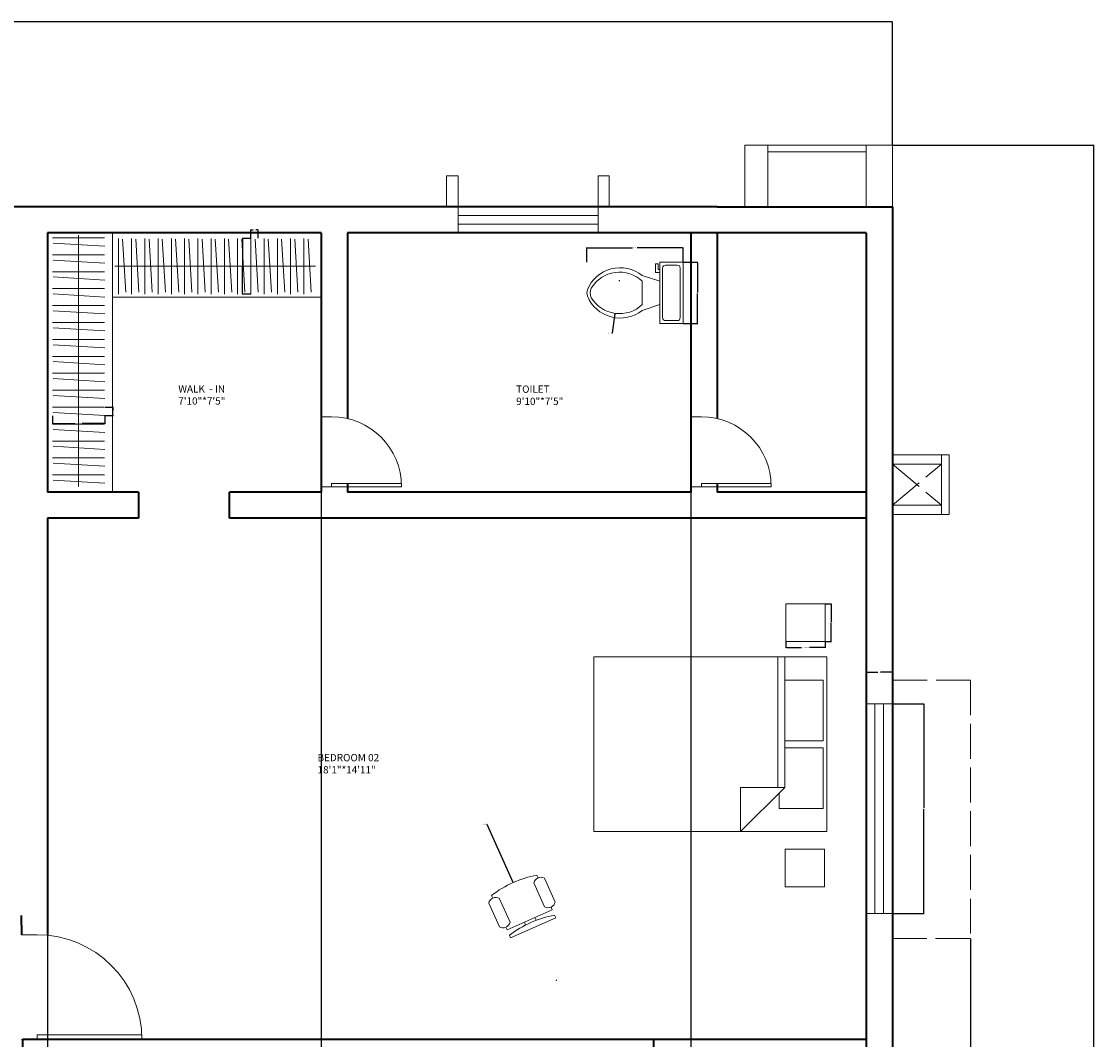
# Model space of a CAD drawing. Units: inches. Extents: x 293720 to 590083, y 155482 to 312405.
# Tile 4 of 4: x 294173 to 294542, y 156028 to 156378. Entities that reach past the tile are written whole.
import ezdxf

# ---------------------------------------------------------------- set-up
doc = ezdxf.new("R2010")
doc.units = ezdxf.units.IN
doc.linetypes.add('ACAD_ISO02W100', pattern=[15, 12, -3])
for name, color, linetype, lineweight in [('A-ANNO-DIMS', 2, 'Continuous', 18), ('A-AREA-IDEN', 7, 'Continuous', 18), ('A-DOOR', 3, 'Continuous', 18), ('A-FLOR-CASE', 8, 'Continuous', 18), ('A-FLOR-FIXT', 9, 'Continuous', 18), ('A-FLOR-OPEN', 8, 'ACAD_ISO02W100', 13), ('A-FLOR-OVHD', 8, 'ACAD_ISO02W100', 13), ('A-FLOR-PROJ', 8, 'Continuous', 18), ('A-FURN', 8, 'Continuous', 18), ('A-GLAZ', 4, 'Continuous', 18), ('A-WALL', 7, 'Continuous', 35)]:
    doc.layers.add(name, color=color, linetype=linetype, lineweight=lineweight)
doc.styles.get("Standard").update_dxf_attribs({"font": 'arial.ttf'})
doc.dimstyles.get("Standard").update_dxf_attribs({"dimtxt": 0.18, "dimasz": 0.18, "dimexe": 0.18, "dimexo": 0.0625, "dimgap": 0.09, "dimtad": 0, "dimtih": 1, "dimtoh": 1, "dimdec": 4, "dimzin": 0, "dimdsep": 46, "dimtxsty": 'Standard', "dimcen": 0.09, "dimadec": 0, "dimazin": 0, "dimtfac": 1, "dimtdec": 4, "dimtofl": 0, "dimtmove": 0, "dimatfit": 3, "dimfxl": 1, "dimtolj": 1, "dimtzin": 0, "dimarcsym": 0})

# ---------------------------------------------------------------- blocks, each defined once
blk = doc.blocks.new('Bed - Queen')
for p, q in [((0, -80.00003), (0, 0)), ((0, 0), (59.99999, 0)), ((59.99999, 0), (59.99999, -80.00003)), ((7.99999, -1.2), (28.79998, -1.2)), ((7.99999, -14.4), (7.99999, -1.2)), ((28.79998, -1.2), (28.79998, -14.4)), ((31.19999, -1.2), (51.99999, -1.2)), ((31.19999, -14.4), (31.19999, -1.2)), ((51.99999, -1.2), (51.99999, -16.4)), ((0, -14.4), (44.8, -14.4)), ((59.99999, -29.6), (44.8, -14.4)), ((44.8, -14.4), (44.8, -29.6)), ((44.8, -16.8), (0, -16.8)), ((51.99999, -16.4), (46.79936, -16.4)), ((44.8, -29.6), (59.99999, -29.6)), ((59.99999, -80.00003), (0, -80.00003))]:
    blk.add_line(p, q)
blk = doc.blocks.new('Toilet - top')
for p, q in [((9.5, -6), (9.5, -2)), ((-10, -8.5), (-8, -8.5)), ((-10, -9.5), (-10, -8.5)), ((-7, -9.5), (-10, -9.5)), ((-8, -8.5), (-8, -8)), ((-7, -8), (-7, -9.5)), ((-4, -8), (-6, -14)), ((4, -8), (6, -14)), ((4, -14), (-4, -14))]:
    blk.add_line(p, q)
blk.add_lwpolyline([(10.5, -8), (10.5, 0), (-10.5, 0), (-10.5, -8)], close=True)
for points in [[(-9.5, -2), (-9.5, -6)], [(8.5, -1), (-8.5, -1)], [(-8.5, -7), (8.5, -7)]]:
    blk.add_lwpolyline(points)
for centre, radius, start, end in [((-8.62, -1.88), 0.884, 81.8699, 188.1301), ((8.62, -1.88), 0.884, 351.8699, 98.1301), ((-8.62, -6.12), 0.884, 171.8699, 278.1301), ((8.62, -6.12), 0.884, 261.8699, 8.1301), ((3.52, -21.58), 12.17, 141.4691, 247.9714), ((4.2, -21.82), 11.33, 136.3677, 238.9468), ((-3.52, -21.58), 12.17, 292.0284, 38.5307), ((-4.2, -21.82), 11.33, 301.053, 43.6321), ((0, -27.88), 4, 245.7318, 294.2682), ((0, -29), 4, 254.8605, 285.1395)]:
    blk.add_arc(centre, radius, start, end)
blk = doc.blocks.new('Chair - Desk')
for p, q in [((-8.5, 0), (-8.5, -1)), ((-8.5, 0), (8.5, 0)), ((8.5, 0), (8.5, -1)), ((-8.5, -3), (-8.5, -4)), ((-8.5, -3), (8.5, -3)), ((-2, -3), (-2, -1.9355)), ((2, -1.9576), (2, -3)), ((8.5, -3), (8.5, -4)), ((-10.5, -5), (-10.5, -14)), ((-6.5, -14), (-6.5, -5)), ((6.5, -5), (6.5, -14)), ((10.5, -14), (10.5, -5)), ((-8.5, -15), (-8.5, -16)), ((8.5, -15), (8.5, -16))]:
    blk.add_line(p, q)
for centre, radius, start, end in [((0, 34.625), 36.625, 256.5803, 283.4197), ((-8.5, -6.5), 2.5, 36.8699, 143.1301), ((8.5, -6.5), 2.5, 36.8699, 143.1301), ((-8.5, -12.5), 2.5, 216.8699, 323.1301), ((8.5, -12.5), 2.5, 216.8699, 323.1301), ((0, 19.625), 36.625, 256.5803, 283.4197)]:
    blk.add_arc(centre, radius, start, end)
blk = doc.blocks.new('*U2')
for p, q in [((0, 0), (0, -6)), ((40, 0), (40, -6))]:
    blk.add_line(p, q)
blk.add_lwpolyline([(0, 0), (0, 40), (1.75, 40), (1.75, 0)], close=True)
blk.add_arc((0, 0), 40, 0, 90)
blk = doc.blocks.new('WIN-48IN')
for p, q in [((0, 9), (48, 9)), ((0, 0), (0, 9)), ((48, 9), (48, 0)), ((0, 6), (48, 6)), ((48, 3), (0, 3)), ((48, 0), (0, 0))]:
    blk.add_line(p, q)
blk = doc.blocks.new('WIN-72IN')
for p, q in [((0, 9), (72, 9)), ((0, 0), (0, 9)), ((72, 9), (72, 0)), ((0, 6), (72, 6)), ((72, 3), (0, 3)), ((72, 0), (0, 0))]:
    blk.add_line(p, q)
blk = doc.blocks.new('WARDROBE-HANGER-17P92IN')
for p, q in [((0, 2.88), (17.92, 2.88)), ((0.29, 1.07), (18.07, 0))]:
    blk.add_line(p, q)
blk = doc.blocks.new('WARDROBE-HANGER-19P14IN')
for p, q in [((0, 19.14), (0, 0)), ((1.42, 18.9), (2.5, 0.6))]:
    blk.add_line(p, q)
blk = doc.blocks.new('NIGHTSTAND-RECT')
blk.add_lwpolyline([(0, 12.99), (13.49, 12.99), (13.49, 0), (0, 0)], close=True)
blk = doc.blocks.new('*D31')
at = {"layer": 'A-ANNO-DIMS', "color": 0, "lineweight": -2, "transparency": 16777216}
for p, q in [((294183.76, 156242.17), (294183.76, 156239.34)), ((294201.83, 156242.17), (294201.83, 156239.34)), ((294183.94, 156239.52), (294191.58, 156239.52)), ((294201.65, 156239.52), (294194.01, 156239.52))]:
    blk.add_line(p, q, dxfattribs=at)
at = {"layer": 'A-ANNO-DIMS', "color": 0, "lineweight": 100, "transparency": 16777216}
for points in [[(294183.94, 156239.55), (294183.94, 156239.49), (294183.76, 156239.52)], [(294201.65, 156239.55), (294201.65, 156239.49), (294201.83, 156239.52)]]:
    blk.add_solid(points, dxfattribs=at)
at = {"layer": 'Defpoints', "color": 0, "lineweight": 100, "transparency": 16777216}
for p in [(294183.76, 156242.23), (294201.83, 156242.23), (294201.83, 156239.52)]:
    blk.add_point(p, dxfattribs=at)
at = {"layer": 'A-ANNO-DIMS', "color": 0, "transparency": 16777216, "insert": (294192.8, 156239.52), "char_height": 0.18, "attachment_point": 5}
blk.add_mtext('\\A1;HANGER E 18 TYP.', dxfattribs=at)
blk = doc.blocks.new('*D32')
at = {"layer": 'A-ANNO-DIMS', "color": 0, "lineweight": -2, "transparency": 16777216}
for p, q in [((294201.89, 156245.11), (294204.72, 156245.11)), ((294204.54, 156244.93), (294204.54, 156243.85)), ((294201.89, 156242.23), (294204.72, 156242.23)), ((294204.54, 156242.41), (294204.54, 156243.49))]:
    blk.add_line(p, q, dxfattribs=at)
at = {"layer": 'A-ANNO-DIMS', "color": 0, "lineweight": 100, "transparency": 16777216}
for points in [[(294204.51, 156244.93), (294204.57, 156244.93), (294204.54, 156245.11)], [(294204.51, 156242.41), (294204.57, 156242.41), (294204.54, 156242.23)]]:
    blk.add_solid(points, dxfattribs=at)
at = {"layer": 'Defpoints', "color": 0, "lineweight": 100, "transparency": 16777216}
for p in [(294201.83, 156245.11), (294204.54, 156245.11), (294201.83, 156242.23)]:
    blk.add_point(p, dxfattribs=at)
at = {"layer": 'A-ANNO-DIMS', "color": 0, "transparency": 16777216, "insert": (294204.54, 156243.67), "char_height": 0.18, "attachment_point": 5}
blk.add_mtext('\\A1;3 TYP.', dxfattribs=at)
blk = doc.blocks.new('*D33')
at = {"layer": 'A-ANNO-DIMS', "color": 0, "lineweight": -2, "transparency": 16777216}
for p, q in [((294251.9, 156303.08), (294248.91, 156303.08)), ((294249.09, 156302.9), (294249.09, 156293.7)), ((294249.09, 156284.12), (294249.09, 156293.33)), ((294251.9, 156283.94), (294248.91, 156283.94))]:
    blk.add_line(p, q, dxfattribs=at)
at = {"layer": 'A-ANNO-DIMS', "color": 0, "lineweight": 100, "transparency": 16777216}
for points in [[(294249.06, 156302.9), (294249.12, 156302.9), (294249.09, 156303.08)], [(294249.06, 156284.12), (294249.12, 156284.12), (294249.09, 156283.94)]]:
    blk.add_solid(points, dxfattribs=at)
at = {"layer": 'Defpoints', "color": 0, "lineweight": 100, "transparency": 16777216}
for p in [(294249.09, 156303.08), (294251.96, 156303.08), (294251.96, 156283.94)]:
    blk.add_point(p, dxfattribs=at)
at = {"layer": 'A-ANNO-DIMS', "color": 0, "transparency": 16777216, "insert": (294249.09, 156293.51), "char_height": 0.18, "attachment_point": 5}
blk.add_mtext('\\A1;HANGER F 19 TYP.', dxfattribs=at)
blk = doc.blocks.new('*D34')
at = {"layer": 'A-ANNO-DIMS', "color": 0, "lineweight": -2, "transparency": 16777216}
for p, q in [((294251.96, 156303.14), (294251.96, 156306.13)), ((294252.14, 156305.95), (294252.75, 156305.95)), ((294254.27, 156305.95), (294253.67, 156305.95)), ((294254.45, 156303.14), (294254.45, 156306.13))]:
    blk.add_line(p, q, dxfattribs=at)
at = {"layer": 'A-ANNO-DIMS', "color": 0, "lineweight": 100, "transparency": 16777216}
for points in [[(294252.14, 156305.98), (294252.14, 156305.92), (294251.96, 156305.95)], [(294254.27, 156305.98), (294254.27, 156305.92), (294254.45, 156305.95)]]:
    blk.add_solid(points, dxfattribs=at)
at = {"layer": 'Defpoints', "color": 0, "lineweight": 100, "transparency": 16777216}
for p in [(294251.96, 156303.08), (294254.45, 156305.95), (294254.45, 156303.08)]:
    blk.add_point(p, dxfattribs=at)
at = {"layer": 'A-ANNO-DIMS', "color": 0, "transparency": 16777216, "insert": (294253.21, 156305.95), "char_height": 0.18, "attachment_point": 5}
blk.add_mtext('\\A1;2 TYP.', dxfattribs=at)
blk = doc.blocks.new('*D39')
at = {"layer": 'A-ANNO-DIMS', "color": 0, "lineweight": -2, "transparency": 16777216}
for p, q in [((294472.34, 156143.27), (294483.26, 156143.27)), ((294483.08, 156143.09), (294483.08, 156107.45)), ((294483.08, 156071.45), (294483.08, 156107.09)), ((294472.34, 156071.27), (294483.26, 156071.27))]:
    blk.add_line(p, q, dxfattribs=at)
at = {"layer": 'A-ANNO-DIMS', "color": 0, "lineweight": 100, "transparency": 16777216}
for points in [[(294483.05, 156143.09), (294483.11, 156143.09), (294483.08, 156143.27)], [(294483.05, 156071.45), (294483.11, 156071.45), (294483.08, 156071.27)]]:
    blk.add_solid(points, dxfattribs=at)
at = {"layer": 'Defpoints', "color": 0, "lineweight": 100, "transparency": 16777216}
for p in [(294472.28, 156143.27), (294483.08, 156143.27), (294472.28, 156071.27)]:
    blk.add_point(p, dxfattribs=at)
at = {"layer": 'A-ANNO-DIMS', "color": 0, "transparency": 16777216, "insert": (294483.08, 156107.27), "char_height": 0.18, "attachment_point": 5}
blk.add_mtext('\\A1;WINDOW 72 TYP.', dxfattribs=at)
blk = doc.blocks.new('*D40')
at = {"layer": 'A-ANNO-DIMS', "color": 0, "lineweight": -2, "transparency": 16777216}
for p, q in [((294463.28, 156143.33), (294463.28, 156154.25)), ((294463.46, 156154.07), (294467.32, 156154.07)), ((294472.1, 156154.07), (294468.23, 156154.07)), ((294472.28, 156143.33), (294472.28, 156154.25))]:
    blk.add_line(p, q, dxfattribs=at)
at = {"layer": 'A-ANNO-DIMS', "color": 0, "lineweight": 100, "transparency": 16777216}
for points in [[(294463.46, 156154.1), (294463.46, 156154.04), (294463.28, 156154.07)], [(294472.1, 156154.1), (294472.1, 156154.04), (294472.28, 156154.07)]]:
    blk.add_solid(points, dxfattribs=at)
at = {"layer": 'Defpoints', "color": 0, "lineweight": 100, "transparency": 16777216}
for p in [(294463.28, 156154.07), (294463.28, 156143.27), (294472.28, 156143.27)]:
    blk.add_point(p, dxfattribs=at)
at = {"layer": 'A-ANNO-DIMS', "color": 0, "transparency": 16777216, "insert": (294467.78, 156154.07), "char_height": 0.18, "attachment_point": 5}
blk.add_mtext('\\A1;9 TYP.', dxfattribs=at)
blk = doc.blocks.new('*D45')
at = {"layer": 'A-ANNO-DIMS', "color": 0, "lineweight": -2, "transparency": 16777216}
for p, q in [((294367.33, 156294.91), (294367.33, 156299.99)), ((294367.51, 156299.81), (294383.08, 156299.81)), ((294400.2, 156299.81), (294384.63, 156299.81)), ((294400.38, 156294.91), (294400.38, 156299.99))]:
    blk.add_line(p, q, dxfattribs=at)
at = {"layer": 'A-ANNO-DIMS', "color": 0, "lineweight": 100, "transparency": 16777216}
for points in [[(294367.51, 156299.84), (294367.51, 156299.78), (294367.33, 156299.81)], [(294400.2, 156299.84), (294400.2, 156299.78), (294400.38, 156299.81)]]:
    blk.add_solid(points, dxfattribs=at)
at = {"layer": 'Defpoints', "color": 0, "lineweight": 100, "transparency": 16777216}
for p in [(294400.38, 156299.81), (294367.33, 156294.85), (294400.38, 156294.85)]:
    blk.add_point(p, dxfattribs=at)
at = {"layer": 'A-ANNO-DIMS', "color": 0, "transparency": 16777216, "insert": (294383.86, 156299.81), "char_height": 0.18, "attachment_point": 5}
blk.add_mtext('\\A1;WC 33 TYP.', dxfattribs=at)
blk = doc.blocks.new('*D46')
at = {"layer": 'A-ANNO-DIMS', "color": 0, "lineweight": -2, "transparency": 16777216}
for p, q in [((294400.44, 156294.85), (294405.52, 156294.85)), ((294405.34, 156294.67), (294405.34, 156284.53)), ((294405.34, 156274.03), (294405.34, 156284.17)), ((294400.44, 156273.85), (294405.52, 156273.85))]:
    blk.add_line(p, q, dxfattribs=at)
at = {"layer": 'A-ANNO-DIMS', "color": 0, "lineweight": 100, "transparency": 16777216}
for points in [[(294405.31, 156294.67), (294405.37, 156294.67), (294405.34, 156294.85)], [(294405.31, 156274.03), (294405.37, 156274.03), (294405.34, 156273.85)]]:
    blk.add_solid(points, dxfattribs=at)
at = {"layer": 'Defpoints', "color": 0, "lineweight": 100, "transparency": 16777216}
for p in [(294400.38, 156294.85), (294400.38, 156273.85), (294405.34, 156273.85)]:
    blk.add_point(p, dxfattribs=at)
at = {"layer": 'A-ANNO-DIMS', "color": 0, "transparency": 16777216, "insert": (294405.34, 156284.35), "char_height": 0.18, "attachment_point": 5}
blk.add_mtext('\\A1;21 TYP.', dxfattribs=at)
blk = doc.blocks.new('*D47')
at = {"layer": 'A-ANNO-DIMS', "color": 0, "lineweight": -2, "transparency": 16777216}
for p, q in [((294435.7, 156164.56), (294435.7, 156162.42)), ((294435.88, 156162.6), (294441.07, 156162.6)), ((294449.02, 156162.6), (294443.83, 156162.6)), ((294449.2, 156164.56), (294449.2, 156162.42))]:
    blk.add_line(p, q, dxfattribs=at)
at = {"layer": 'A-ANNO-DIMS', "color": 0, "lineweight": 100, "transparency": 16777216}
for points in [[(294435.88, 156162.63), (294435.88, 156162.57), (294435.7, 156162.6)], [(294449.02, 156162.63), (294449.02, 156162.57), (294449.2, 156162.6)]]:
    blk.add_solid(points, dxfattribs=at)
at = {"layer": 'Defpoints', "color": 0, "lineweight": 100, "transparency": 16777216}
for p in [(294435.7, 156164.63), (294449.2, 156164.63), (294449.2, 156162.6)]:
    blk.add_point(p, dxfattribs=at)
at = {"layer": 'A-ANNO-DIMS', "color": 0, "transparency": 16777216, "insert": (294442.45, 156162.6), "char_height": 0.18, "attachment_point": 5}
blk.add_mtext('\\A1;NIGHTSTAND 13 TYP.', dxfattribs=at)
blk = doc.blocks.new('*D48')
at = {"layer": 'A-ANNO-DIMS', "color": 0, "lineweight": -2, "transparency": 16777216}
for p, q in [((294449.26, 156177.61), (294451.4, 156177.61)), ((294451.22, 156177.43), (294451.22, 156171.3)), ((294451.22, 156164.81), (294451.22, 156170.94)), ((294449.26, 156164.63), (294451.4, 156164.63))]:
    blk.add_line(p, q, dxfattribs=at)
at = {"layer": 'A-ANNO-DIMS', "color": 0, "lineweight": 100, "transparency": 16777216}
for points in [[(294451.19, 156177.43), (294451.25, 156177.43), (294451.22, 156177.61)], [(294451.19, 156164.81), (294451.25, 156164.81), (294451.22, 156164.63)]]:
    blk.add_solid(points, dxfattribs=at)
at = {"layer": 'Defpoints', "color": 0, "lineweight": 100, "transparency": 16777216}
for p in [(294449.2, 156177.61), (294451.22, 156177.61), (294449.2, 156164.63)]:
    blk.add_point(p, dxfattribs=at)
at = {"layer": 'A-ANNO-DIMS', "color": 0, "transparency": 16777216, "insert": (294451.22, 156171.12), "char_height": 0.18, "attachment_point": 5}
blk.add_mtext('\\A1;13 TYP.', dxfattribs=at)
blk = doc.blocks.new('*D53')
at = {"layer": 'A-ANNO-DIMS', "color": 0, "lineweight": -2, "transparency": 16777216}
for p, q in [((294499.07, 156062.55), (294499.07, 155481.85)), ((293762.89, 155594.88), (293762.89, 155481.85)), ((293763.07, 155482.03), (294130.59, 155482.03)), ((294498.89, 155482.03), (294131.37, 155482.03))]:
    blk.add_line(p, q, dxfattribs=at)
at = {"layer": 'A-ANNO-DIMS', "color": 0, "lineweight": 100, "transparency": 16777216}
for points in [[(293763.07, 155482.06), (293763.07, 155482), (293762.89, 155482.03)], [(294498.89, 155482.06), (294498.89, 155482), (294499.07, 155482.03)]]:
    blk.add_solid(points, dxfattribs=at)
at = {"layer": 'Defpoints', "color": 0, "lineweight": 100, "transparency": 16777216}
for p in [(294499.07, 156062.61), (293762.89, 155594.94), (294499.07, 155482.03)]:
    blk.add_point(p, dxfattribs=at)
at = {"layer": 'A-ANNO-DIMS', "color": 0, "transparency": 16777216, "insert": (294130.98, 155482.03), "char_height": 0.18, "attachment_point": 5}
blk.add_mtext('\\A1;736.2', dxfattribs=at)
blk = doc.blocks.new('*D54')
at = {"layer": 'A-ANNO-DIMS', "color": 0, "lineweight": -2, "transparency": 16777216}
for p, q in [((294472.34, 156335.04), (294541.6, 156335.04)), ((294541.42, 156334.86), (294541.42, 155929.89)), ((294541.42, 155524.56), (294541.42, 155929.53)), ((294472.34, 155524.38), (294541.6, 155524.38))]:
    blk.add_line(p, q, dxfattribs=at)
at = {"layer": 'A-ANNO-DIMS', "color": 0, "lineweight": 100, "transparency": 16777216}
for points in [[(294541.39, 156334.86), (294541.45, 156334.86), (294541.42, 156335.04)], [(294541.39, 155524.56), (294541.45, 155524.56), (294541.42, 155524.38)]]:
    blk.add_solid(points, dxfattribs=at)
at = {"layer": 'Defpoints', "color": 0, "lineweight": 100, "transparency": 16777216}
for p in [(294472.28, 156335.04), (294541.42, 156335.04), (294472.28, 155524.38)]:
    blk.add_point(p, dxfattribs=at)
at = {"layer": 'A-ANNO-DIMS', "color": 0, "transparency": 16777216, "insert": (294541.42, 155929.71), "char_height": 0.18, "attachment_point": 5}
blk.add_mtext('\\A1;810.7', dxfattribs=at)
blk = doc.blocks.new('*D55')
at = {"layer": 'A-ANNO-DIMS', "color": 0, "lineweight": -2, "transparency": 16777216}
for p, q in [((293803.09, 156313.99), (293803.09, 156377.57)), ((293803.27, 156377.39), (294137.29, 156377.39)), ((294472.1, 156377.39), (294138.08, 156377.39)), ((294472.28, 156335.1), (294472.28, 156377.57))]:
    blk.add_line(p, q, dxfattribs=at)
at = {"layer": 'A-ANNO-DIMS', "color": 0, "lineweight": 100, "transparency": 16777216}
for points in [[(293803.27, 156377.42), (293803.27, 156377.36), (293803.09, 156377.39)], [(294472.1, 156377.42), (294472.1, 156377.36), (294472.28, 156377.39)]]:
    blk.add_solid(points, dxfattribs=at)
at = {"layer": 'Defpoints', "color": 0, "lineweight": 100, "transparency": 16777216}
for p in [(294472.28, 156377.39), (294472.28, 156335.04), (293803.09, 156313.93)]:
    blk.add_point(p, dxfattribs=at)
at = {"layer": 'A-ANNO-DIMS', "color": 0, "transparency": 16777216, "insert": (294137.68, 156377.39), "char_height": 0.18, "attachment_point": 5}
blk.add_mtext('\\A1;669.2', dxfattribs=at)
blk = doc.blocks.new('*D59')
at = {"layer": 'A-ANNO-DIMS', "color": 0, "lineweight": -2, "transparency": 16777216}
for p, q in [((294276.09, 156215.87), (294276.09, 155481.85)), ((294182.09, 156206.87), (294182.09, 155481.85)), ((294182.27, 155482.03), (294228.87, 155482.03)), ((294275.91, 155482.03), (294229.31, 155482.03))]:
    blk.add_line(p, q, dxfattribs=at)
at = {"layer": 'A-ANNO-DIMS', "color": 0, "lineweight": 100, "transparency": 16777216}
for points in [[(294182.27, 155482.06), (294182.27, 155482), (294182.09, 155482.03)], [(294275.91, 155482.06), (294275.91, 155482), (294276.09, 155482.03)]]:
    blk.add_solid(points, dxfattribs=at)
at = {"layer": 'Defpoints', "color": 0, "lineweight": 100, "transparency": 16777216}
for p in [(294276.09, 156215.93), (294182.09, 156206.93), (294276.09, 155482.03)]:
    blk.add_point(p, dxfattribs=at)
at = {"layer": 'A-ANNO-DIMS', "color": 0, "transparency": 16777216, "insert": (294229.09, 155482.03), "char_height": 0.18, "attachment_point": 5}
blk.add_mtext('\\A1;94', dxfattribs=at)
blk = doc.blocks.new('*D60')
at = {"layer": 'A-ANNO-DIMS', "color": 0, "lineweight": -2, "transparency": 16777216}
for p, q in [((294276.09, 156215.87), (294276.09, 155481.85)), ((294403.09, 156215.87), (294403.09, 155481.85)), ((294276.27, 155482.03), (294339.31, 155482.03)), ((294402.91, 155482.03), (294339.87, 155482.03))]:
    blk.add_line(p, q, dxfattribs=at)
at = {"layer": 'A-ANNO-DIMS', "color": 0, "lineweight": 100, "transparency": 16777216}
for points in [[(294276.27, 155482.06), (294276.27, 155482), (294276.09, 155482.03)], [(294402.91, 155482.06), (294402.91, 155482), (294403.09, 155482.03)]]:
    blk.add_solid(points, dxfattribs=at)
at = {"layer": 'Defpoints', "color": 0, "lineweight": 100, "transparency": 16777216}
for p in [(294276.09, 156215.93), (294403.09, 156215.93), (294403.09, 155482.03)]:
    blk.add_point(p, dxfattribs=at)
at = {"layer": 'A-ANNO-DIMS', "color": 0, "transparency": 16777216, "insert": (294339.59, 155482.03), "char_height": 0.18, "attachment_point": 5}
blk.add_mtext('\\A1;127', dxfattribs=at)
blk = doc.blocks.new('*D76')
at = {"layer": 'A-ANNO-DIMS', "color": 0, "lineweight": -2, "transparency": 16777216}
for p, q in [((294332.86, 156101.88), (294333.04, 156101.88)), ((294333.04, 156101.88), (294341.93, 156081.98)), ((294356.84, 156048.37), (294357.02, 156048.37)), ((294356.93, 156048.28), (294356.93, 156048.46))]:
    blk.add_line(p, q, dxfattribs=at)
at = {"layer": 'A-ANNO-DIMS', "color": 0, "lineweight": 100, "transparency": 16777216}
blk.add_solid([(294341.95, 156081.99), (294341.9, 156081.97), (294342, 156081.82)], dxfattribs=at)
at = {"layer": 'Defpoints', "color": 0, "lineweight": 100, "transparency": 16777216}
for p in [(294342, 156081.82), (294356.93, 156048.37)]:
    blk.add_point(p, dxfattribs=at)
at = {"layer": 'A-ANNO-DIMS', "color": 0, "transparency": 16777216, "insert": (294332.06, 156101.88), "char_height": 0.18, "attachment_point": 5}
blk.add_mtext('\\A1;10X R36.625', dxfattribs=at)
blk = doc.blocks.new('*D82')
at = {"layer": 'A-ANNO-DIMS', "color": 0, "lineweight": -2, "transparency": 16777216}
for p, q in [((294378.47, 156288.55), (294378.65, 156288.55)), ((294378.56, 156288.46), (294378.56, 156288.64)), ((294376.15, 156270.58), (294377.03, 156277.14)), ((294375.97, 156270.58), (294376.15, 156270.58))]:
    blk.add_line(p, q, dxfattribs=at)
at = {"layer": 'A-ANNO-DIMS', "color": 0, "lineweight": 100, "transparency": 16777216}
blk.add_solid([(294377, 156277.15), (294377.06, 156277.14), (294377.05, 156277.32)], dxfattribs=at)
at = {"layer": 'Defpoints', "color": 0, "lineweight": 100, "transparency": 16777216}
for p in [(294378.56, 156288.55), (294377.05, 156277.32)]:
    blk.add_point(p, dxfattribs=at)
at = {"layer": 'A-ANNO-DIMS', "color": 0, "transparency": 16777216, "insert": (294375.29, 156270.58), "char_height": 0.18, "attachment_point": 5}
blk.add_mtext('\\A1;6X R11.33', dxfattribs=at)

msp = doc.modelspace()

# ---------------------------------------------------------------- linework, layer by layer
at = {"layer": 'A-FLOR-CASE'}
for p, q in [((294192.7245, 156304.1988), (294192.7245, 156217.8367)), ((294204.4036, 156282.8656), (294204.4036, 156304.9282)), ((294206.4487, 156293.5128), (294205.2043, 156293.5128)), ((294206.4487, 156293.5128), (294274.2052, 156293.5128)), ((294204.4036, 156215.8788), (294204.4036, 156282.8656)), ((294204.4036, 156282.8656), (294276.0931, 156282.8656))]:
    msp.add_line(p, q, dxfattribs=at)
at = {"layer": 'A-FLOR-OPEN'}
for p, q in [((294472.2763, 156225.5073), (294489.1768, 156211.4983)), ((294472.2763, 156211.4983), (294489.1768, 156225.5073))]:
    msp.add_line(p, q, dxfattribs=at)
at = {"layer": 'A-FLOR-OVHD'}
for p, q in [((294472.2763, 156151.3058), (294499.0676, 156151.3058)), ((294499.0676, 156151.3058), (294499.0676, 156062.6102)), ((294499.0676, 156062.6102), (294472.2763, 156062.6102))]:
    msp.add_line(p, q, dxfattribs=at)
at = {"layer": 'A-FLOR-PROJ'}
for p, q in [((294429.4997, 156335.0376), (294421.5739, 156335.0376)), ((294421.5739, 156335.0376), (294421.5739, 156313.9282)), ((294429.4997, 156313.9282), (294429.4997, 156335.0376)), ((294429.4997, 156335.0376), (294463.2763, 156335.0376)), ((294429.4997, 156332.7769), (294463.2763, 156332.7769)), ((294472.2763, 156335.0376), (294463.2763, 156335.0376)), ((294463.2763, 156335.0376), (294463.2763, 156313.9282)), ((294472.2763, 156313.9282), (294472.2763, 156335.0376)), ((294323.1955, 156324.5735), (294319.14, 156324.5735)), ((294319.14, 156324.5735), (294319.14, 156313.9282)), ((294323.1955, 156313.9282), (294323.1955, 156324.5735)), ((294371.1955, 156324.5735), (294371.1955, 156313.9282)), ((294371.1955, 156324.5735), (294375.0662, 156324.5735)), ((294375.0662, 156324.5735), (294375.0662, 156313.9282)), ((294489.1768, 156228.7206), (294472.2763, 156228.7206)), ((294472.2763, 156225.5073), (294489.1768, 156225.5073)), ((294489.1768, 156225.5073), (294489.1768, 156228.7206)), ((294489.1768, 156228.7206), (294491.7918, 156228.7206)), ((294489.1768, 156225.5073), (294489.1768, 156211.4983)), ((294491.7918, 156228.7206), (294491.7918, 156208.2173)), ((294489.1768, 156211.4983), (294472.2763, 156211.4983)), ((294489.1768, 156208.2173), (294489.1768, 156211.4983)), ((294472.2763, 156208.2173), (294489.1768, 156208.2173)), ((294491.7918, 156208.2173), (294489.1768, 156208.2173))]:
    msp.add_line(p, q, dxfattribs=at)
at = {"layer": 'A-WALL'}
for p, q in [((294412.0931, 156313.9282), (293803.0931, 156313.9282)), ((294412.0931, 156313.9282), (294472.2763, 156313.9282)), ((294472.2763, 156313.9282), (294472.2763, 155990.6883)), ((294182.0931, 156304.9282), (294182.0931, 156215.9282)), ((294276.0931, 156304.9282), (294182.0931, 156304.9282)), ((294276.0931, 156304.9282), (294276.0931, 156215.9282)), ((294463.2763, 156304.9282), (294285.0931, 156304.9282)), ((294285.0931, 156304.9282), (294285.0931, 156241.1679)), ((294403.0931, 156304.9282), (294403.0931, 156215.9282)), ((294412.0931, 156304.9282), (294412.0931, 156241.1679)), ((294463.2763, 156304.9282), (294463.2763, 155954.9282)), ((294285.0931, 156218.8332), (294285.0931, 156215.9282)), ((294412.0931, 156218.8332), (294412.0931, 156215.9282)), ((294213.3829, 156215.8589), (294182.0931, 156215.9282)), ((294213.3829, 156215.8589), (294213.3829, 156206.9282)), ((294244.5632, 156206.9282), (294244.5632, 156215.9282)), ((294276.0931, 156215.9282), (294244.5632, 156215.9282)), ((294403.0931, 156215.9282), (294285.0931, 156215.9282)), ((294463.2763, 156215.9282), (294412.0931, 156215.9282)), ((294213.3829, 156206.9282), (294182.0931, 156206.9282)), ((294182.0931, 156206.9282), (294182.0931, 156063.754)), ((294463.2763, 156206.9282), (294244.5632, 156206.9282)), ((294173.0931, 156070.5313), (294173.1558, 156063.9282)), ((294463.2763, 156027.9282), (294173.4975, 156027.9282)), ((294173.4975, 156027.9282), (294173.4975, 156018.9282)), ((294390.2763, 156027.9282), (294390.2763, 155954.9282))]:
    msp.add_line(p, q, dxfattribs=at)

# ---------------------------------------------------------------- block references
at = {"layer": 'A-DOOR', "rotation": 270}
for p, xscale, yscale, zscale in [((294279.6931, 156217.7832), -0.6, 0.6, 0.6), ((294406.6931, 156217.7832), -0.6, 0.6, 0.6), ((294178.5558, 156027.9282), -0.9, 0.9, 0.9)]:
    msp.add_blockref('*U2', p, dxfattribs=dict(at, xscale=xscale, yscale=yscale, zscale=zscale))
at = {"layer": 'A-FLOR-CASE'}
for name, p in [('WARDROBE-HANGER-17P92IN', (294183.765, 156300.372)), ('WARDROBE-HANGER-19P14IN', (294206.449, 156283.944)), ('WARDROBE-HANGER-19P14IN', (294211, 156283.944)), ('WARDROBE-HANGER-19P14IN', (294215.5511, 156283.944)), ('WARDROBE-HANGER-19P14IN', (294220.1021, 156283.944)), ('WARDROBE-HANGER-19P14IN', (294224.6531, 156283.944)), ('WARDROBE-HANGER-19P14IN', (294229.2042, 156283.944)), ('WARDROBE-HANGER-19P14IN', (294233.7552, 156283.944)), ('WARDROBE-HANGER-19P14IN', (294238.3062, 156283.944)), ('WARDROBE-HANGER-19P14IN', (294242.8573, 156283.944)), ('WARDROBE-HANGER-19P14IN', (294247.4083, 156283.944)), ('WARDROBE-HANGER-19P14IN', (294251.9594, 156283.944)), ('WARDROBE-HANGER-19P14IN', (294256.5104, 156283.944)), ('WARDROBE-HANGER-19P14IN', (294261.0614, 156283.944)), ('WARDROBE-HANGER-19P14IN', (294265.6125, 156283.944)), ('WARDROBE-HANGER-19P14IN', (294270.1635, 156283.944)), ('WARDROBE-HANGER-17P92IN', (294183.765, 156294.5576)), ('WARDROBE-HANGER-17P92IN', (294183.765, 156288.7432)), ('WARDROBE-HANGER-17P92IN', (294183.765, 156282.9289)), ('WARDROBE-HANGER-17P92IN', (294183.765, 156277.1145)), ('WARDROBE-HANGER-17P92IN', (294183.765, 156271.3001)), ('WARDROBE-HANGER-17P92IN', (294183.765, 156265.4857)), ('WARDROBE-HANGER-17P92IN', (294183.765, 156259.6714)), ('WARDROBE-HANGER-17P92IN', (294183.765, 156253.857)), ('WARDROBE-HANGER-17P92IN', (294183.765, 156248.0426)), ('WARDROBE-HANGER-17P92IN', (294183.765, 156242.2282)), ('WARDROBE-HANGER-17P92IN', (294183.765, 156236.4139)), ('WARDROBE-HANGER-17P92IN', (294183.765, 156230.5995)), ('WARDROBE-HANGER-17P92IN', (294183.765, 156224.7851)), ('WARDROBE-HANGER-17P92IN', (294183.765, 156218.9707))]:
    msp.add_blockref(name, p, dxfattribs=at)
at = {"layer": 'A-FLOR-FIXT', "rotation": 270}
msp.add_blockref('Toilet - top', (294400.381, 156284.3489), dxfattribs=at)
at = {"layer": 'A-FURN'}
for p in [(294435.703, 156164.625), (294435.5065, 156080.3603)]:
    msp.add_blockref('NIGHTSTAND-RECT', p, dxfattribs=at)
for name, p, rotation in [('Bed - Queen', (294449.7698, 156159.3275), 270), ('Chair - Desk', (294348.9283, 156066.2934), 204.0552673600429)]:
    msp.add_blockref(name, p, dxfattribs=dict(at, rotation=rotation))
at = {"layer": 'A-GLAZ'}
msp.add_blockref('WIN-48IN', (294323.1958, 156304.928), dxfattribs=at)
at = {"layer": 'A-GLAZ', "rotation": 90.0000000000912}
msp.add_blockref('WIN-72IN', (294472.2765, 156071.2685), dxfattribs=at)

# ---------------------------------------------------------------- texts
at = {"layer": 'A-AREA-IDEN', "char_height": 2.5, "attachment_point": 1}
for s, width, insert in [('WALK  - IN\\P7\'10"*7\'5"', 47.101275, (294227.0152, 156252.6401)), ('TOILET\\P9\'10"*7\'5"', 53.118509, (294343.0796, 156252.5457)), ('BEDROOM 02\\P18\'1"*14\'11"', 89.240388, (294274.8565, 156125.9893))]:
    msp.add_mtext_dynamic_manual_height_columns(s, width=width, gutter_width=12.5, heights=[0], dxfattribs=dict(at, insert=insert))

# ---------------------------------------------------------------- dimensions: what is measured, and where the dimension line sits
at = {"layer": 'A-ANNO-DIMS'}
for base, p1, p2, override, picture, middle in [((294472.2763, 156377.3876), (293803.0931, 156313.9282), (294472.2763, 156335.0376), {"dimdec": 1, "dimlfac": 1, "dimrnd": 0, "dimzin": 0, "dimdsep": 46, "dimlunit": 2}, '*D55', (294137.6847, 156377.3876)), ((294276.0931, 155482.0334), (294182.0931, 156206.9282), (294276.0931, 156215.9282), {"dimdec": 0, "dimlfac": 1, "dimrnd": 0, "dimzin": 0, "dimdsep": 46, "dimlunit": 2}, '*D59', (294229.0931, 155482.0334)), ((294403.0931, 155482.0334), (294276.0931, 156215.9282), (294403.0931, 156215.9282), {"dimdec": 0, "dimlfac": 1, "dimrnd": 0, "dimzin": 0, "dimdsep": 46, "dimlunit": 2}, '*D60', (294339.5931, 155482.0334)), ((294499.0676, 155482.0334), (293762.8891, 155594.9386), (294499.0676, 156062.6102), {"dimdec": 1, "dimlfac": 1, "dimrnd": 0, "dimzin": 0, "dimdsep": 46, "dimlunit": 2}, '*D53', (294130.9783, 155482.0334))]:
    dim = msp.add_linear_dim(base=base, p1=p1, p2=p2, dimstyle='Standard', override=override, dxfattribs=at)
    dim.commit()
    dim.dimension.update_dxf_attribs({"geometry": picture, "text_midpoint": middle})
dim = msp.add_linear_dim(base=(294541.4176, 156335.0376), p1=(294472.2763, 155524.3834), p2=(294472.2763, 156335.0376), angle=90, dimstyle='Standard', override={"dimdec": 1, "dimlfac": 1, "dimrnd": 0, "dimzin": 0, "dimdsep": 46, "dimlunit": 2}, dxfattribs=at)
dim.commit()
dim.dimension.update_dxf_attribs({"geometry": '*D54', "text_midpoint": (294541.4176, 155929.7105)})
for base, p1, p2, text, picture, middle in [((294254.4545, 156305.9527), (294251.9591, 156303.0819), (294254.4545, 156303.0819), '<> TYP.', '*D34', (294253.2068, 156305.9527)), ((294400.381, 156299.8058), (294367.3348, 156294.8489), (294400.381, 156294.8489), 'WC <> TYP.', '*D45', (294383.8579, 156299.8058)), ((294201.8312, 156239.518), (294183.7647, 156242.228), (294201.8312, 156242.228), 'HANGER E <> TYP.', '*D31', (294192.7979, 156239.518)), ((294449.1978, 156162.6013), (294435.703, 156164.6255), (294449.1978, 156164.6255), 'NIGHTSTAND <> TYP.', '*D47', (294442.4504, 156162.6013))]:
    dim = msp.add_linear_dim(base=base, p1=p1, p2=p2, text=text, dimstyle='Standard', override={"dimdec": 0, "dimlfac": 1, "dimrnd": 0, "dimzin": 0, "dimdsep": 46, "dimlunit": 2}, dxfattribs=at)
    dim.commit()
    dim.dimension.update_dxf_attribs({"geometry": picture, "text_midpoint": middle})
for base, p1, p2, angle, text, picture, middle in [((294249.0883, 156303.0819), (294251.9591, 156283.9436), (294251.9591, 156303.0819), 90, 'HANGER F <> TYP.', '*D33', (294249.0883, 156293.5128)), ((294405.338, 156273.8489), (294400.381, 156294.8489), (294400.381, 156273.8489), 270, '<> TYP.', '*D46', (294405.338, 156284.3489)), ((294204.5412, 156245.1065), (294201.8312, 156242.228), (294201.8312, 156245.1065), 90, '<> TYP.', '*D32', (294204.5412, 156243.6672)), ((294451.2221, 156177.6108), (294449.1978, 156164.6255), (294449.1978, 156177.6108), 90, '<> TYP.', '*D48', (294451.2221, 156171.1181)), ((294463.2763, 156154.0682), (294472.2763, 156143.2682), (294463.2763, 156143.2682), 180, '<> TYP.', '*D40', (294467.7763, 156154.0682)), ((294483.0763, 156143.2682), (294472.2763, 156071.2682), (294472.2763, 156143.2682), 90, 'WINDOW <> TYP.', '*D39', (294483.0763, 156107.2682))]:
    dim = msp.add_linear_dim(base=base, p1=p1, p2=p2, angle=angle, text=text, dimstyle='Standard', override={"dimdec": 0, "dimlfac": 1, "dimrnd": 0, "dimzin": 0, "dimdsep": 46, "dimlunit": 2}, dxfattribs=at)
    dim.commit()
    dim.dimension.update_dxf_attribs({"geometry": picture, "text_midpoint": middle})
for center, mpoint, text, override, picture, middle in [((294378.5637, 156288.5488), (294377.054, 156277.3207), '6X <>', {"dimdec": 2, "dimlfac": 1, "dimrnd": 0, "dimzin": 0, "dimdsep": 46, "dimlunit": 2}, '*D82', (294375.2944, 156270.5838)), ((294356.9278, 156048.3728), (294341.999, 156081.8171), '10X <>', {"dimdec": 3, "dimlfac": 1, "dimrnd": 0, "dimzin": 0, "dimdsep": 46, "dimlunit": 2}, '*D76', (294332.0564, 156101.8837))]:
    dim = msp.add_radius_dim(center=center, mpoint=mpoint, text=text, dimstyle='Standard', override=override, dxfattribs=at)
    dim.commit()
    dim.dimension.update_dxf_attribs({"geometry": picture, "text_midpoint": middle, "dimtype": 164})

doc.saveas('drawing.dxf')
